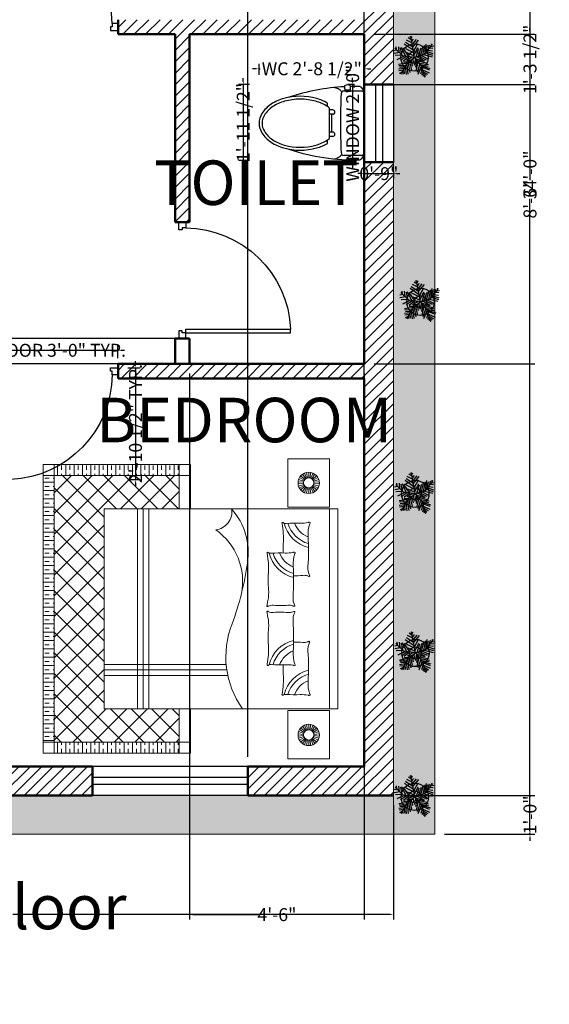
# Model space of a CAD drawing. Units: inches. Extents: x 1265938 to 1266301, y 2357745 to 2358240.
# Tile 2 of 4: x 1266131 to 1266295, y 2357745 to 2358050. Entities that reach past the tile are written whole.
import ezdxf

# ---------------------------------------------------------------- set-up
doc = ezdxf.new("R2010")
doc.units = ezdxf.units.IN
doc.header["$MEASUREMENT"] = 0
for name, color, linetype, lineweight in [('A-ANNO-TEXT', 7, 'Continuous', 25), ('A-AREA-IDEN', 7, 'Continuous', 18), ('A-DOOR', 4, 'Continuous', 25), ('A-FLOR-FIXT', 9, 'Continuous', 25), ('A-FURN', 8, 'Continuous', 18), ('A-WALL-PATT', 8, 'Continuous', 13), ('L-PLNT', 3, 'Continuous', 18), ('L-PLNT-BEDS', 3, 'Continuous', 18), ('L-PLNT-PATT', 3, 'Continuous', 13), ('WALL', 7, 'Continuous', 50), ('WINDOW', 2, 'Continuous', 25), ('YQ_DIM', 3, 'Continuous', 18)]:
    doc.layers.add(name, color=color, linetype=linetype, lineweight=lineweight)
doc.layers.add('Layer2', color=102, linetype='Continuous')
doc.layers.add('RAMP SLOPE', color=8, linetype='Continuous')
doc.styles.get("Standard").update_dxf_attribs({"font": 'arial.ttf'})
doc.styles.add('YQ_DIM', font='SUPEROS.SHX', dxfattribs={"width": 0.8, "bigfont": 'HZDX.SHX'})
doc.dimstyles.new('yqi0', dxfattribs={"dimscale": 0, "dimtxt": 4, "dimasz": 1, "dimexe": 1.5, "dimexo": 3, "dimgap": 0.5, "dimtad": 0, "dimdsep": 46, "dimlunit": 4, "dimtxsty": 'Standard', "dimcen": 0, "dimclrd": 256, "dimclre": 256, "dimclrt": 7, "dimadec": 1, "dimazin": 2, "dimtfac": 1, "dimtix": 1, "dimtmove": 2, "dimatfit": 2, "dimfxl": 1, "dimtolj": 1, "dimtzin": 0, "dimarcsym": 0})

# ---------------------------------------------------------------- blocks, each defined once
blk = doc.blocks.new('WD_WIN4')
for p, q in [((-0.5, 0.5), (0.5, 0.5)), ((-0.5, 0.12), (0.5, 0.12)), ((-0.5, -0.12), (0.5, -0.12)), ((-0.5, -0.5), (0.5, -0.5))]:
    blk.add_line(p, q)
blk = doc.blocks.new('DR_D01')
for p, q in [((-0.45, 0.93), (-0.42, 0.93)), ((-0.45, 0.03), (-0.45, 0.93)), ((-0.42, 0.03), (-0.42, 0.93)), ((-0.5, 0.03), (-0.42, 0.03)), ((-0.5, 0.03), (-0.5, -0.03)), ((-0.45, 0.03), (-0.45, 0)), ((-0.45, 0), (-0.435, 0)), ((-0.435, 0), (-0.435, -0.03)), ((0.435, 0), (0.435, -0.03)), ((0.45, 0), (0.435, 0)), ((0.45, 0.03), (0.45, 0)), ((0.5, 0.03), (0.45, 0.03)), ((0.5, -0.03), (0.5, 0.03)), ((-0.435, -0.03), (-0.5, -0.03)), ((0.435, -0.03), (0.5, -0.03))]:
    blk.add_line(p, q)
blk.add_arc((-0.4602, 0.0206), 0.9103, 0.59152, 87.46644)
blk = doc.blocks.new('Trees - Metric')
at = {"layer": 'Layer2'}
for p, q in [((-258.7244, 1362.456), (-332.3336, 1421.4348)), ((0, 0), (-266.7, 1447.8)), ((-231.1146, 1315.2628), (-166.7002, 1421.4348)), ((-1234.059, 536.7274), (-1252.4486, 737.2604)), ((-1105.2302, 725.4494), (-1077.6458, 395.1732)), ((-902.8176, 713.6638), (-617.5756, 100.2538)), ((-93.091, 489.5342), (-700.3796, 902.3858)), ((-129.8956, 713.6638), (-626.7704, 1032.1544)), ((-185.1152, 1008.5578), (-553.1612, 1185.4942)), ((-221.9198, 1197.3052), (-433.5526, 1338.8594)), ((-194.31, 1102.9442), (-65.4812, 1256.284)), ((-148.3106, 914.1968), (118.5418, 1220.9018)), ((-129.8956, 701.8528), (265.7602, 1185.4942)), ((-74.7014, 418.7444), (219.7608, 961.39)), ((-28.6766, 171.0436), (228.9556, 678.2816)), ((412.9786, 147.447), (587.8068, 796.2392)), ((560.197, 182.8292), (698.2206, 819.8358)), ((685.8, 228.6), (1219.2, 914.4)), ((689.0258, 230.0224), (790.2448, 914.1968)), ((808.6344, 784.4282), (827.0494, 418.7444)), ((891.4384, 831.6214), (946.658, 572.1096)), ((983.4626, 867.0036), (1066.2666, 725.4494)), ((1112.2914, 760.8316), (1296.3144, 784.4282)), ((1121.4862, 925.9824), (1149.0706, 831.6214)), ((-1206.4492, 501.3198), (-1418.082, 465.9376)), ((-1031.621, 347.98), (-1399.667, 277.1902)), ((-800.1, 114.3), (-1333.5, 647.7)), ((-847.598, 159.2326), (-1326.0578, 135.636)), ((-718.7946, 88.4682), (-1215.644, -147.447)), ((-976.4268, 666.4706), (-884.4026, 194.6402)), ((-543.9664, 76.6572), (-967.2066, -206.4512)), ((0, 0), (-800.1, 114.3)), ((-369.1382, 53.086), (-783.1836, 642.874)), ((-405.9428, 53.086), (-764.794, -241.8334)), ((-617.5756, 607.4918), (-74.7014, 347.98)), ((0, 0), (-571.5, -495.3)), ((-166.7002, 29.4894), (-543.9664, -206.4512)), ((-525.5514, 347.98), (-28.6766, 123.8504)), ((0, 0), (685.8, 228.6)), ((0, 0), (457.2, -571.5)), ((100.1268, 41.275), (284.1498, 619.2774)), ((164.5412, 41.275), (661.416, -218.2368)), ((256.5654, 88.4682), (449.7832, 666.4706)), ((284.1498, 88.4682), (781.0246, -147.447)), ((458.978, 147.447), (891.4384, -88.4682)), ((615.4166, 194.6402), (1185.8752, 41.275)), ((753.4148, 312.5978), (1222.6798, 159.2326)), ((845.439, 418.7444), (1241.0948, 277.1902)), ((919.0482, 501.3198), (1222.6798, 454.152)), ((1029.462, 654.685), (1241.0948, 631.0884)), ((-442.7474, -383.3876), (-1086.8406, -477.7486)), ((-617.5756, -548.5384), (-1077.6458, -560.324)), ((-681.9646, -666.496), (-1022.4262, -654.685)), ((-571.5, -495.3), (-952.5, -1143)), ((-387.5278, -324.4088), (-764.794, -324.4088)), ((-635.9652, -607.5172), (-580.771, -1150.1374)), ((-525.5514, -465.963), (-451.9422, -1126.5408)), ((-166.7002, -147.447), (-507.1618, -253.619)), ((-433.5526, -383.3876), (-323.1134, -1020.3688)), ((-341.5284, -289.0012), (-221.9198, -831.6214)), ((-240.3094, -218.2368), (-157.5054, -595.7062)), ((-120.7008, -88.4682), (-93.091, -371.5766)), ((63.3222, -76.6826), (-37.8714, -513.1308)), ((44.9326, -64.897), (615.4166, -241.8334)), ((127.7366, -159.258), (54.1274, -654.685)), ((228.9556, -289.0012), (90.932, -914.1968)), ((357.759, -430.5554), (164.5412, -1020.3688)), ((192.151, -230.0224), (817.8292, -371.5766)), ((458.978, -572.1096), (210.5406, -1161.923)), ((311.7596, -383.3876), (937.4378, -477.7486)), ((412.9786, -501.3452), (919.0482, -583.9206)), ((457.2, -571.5), (685.8, -1333.5)), ((468.1982, -572.1096), (1029.462, -737.2604)), ((486.5878, -642.8994), (983.4626, -843.4324)), ((-718.7946, -737.2604), (-1086.8406, -796.2392)), ((-783.1836, -867.029), (-1077.6458, -902.4112)), ((-875.2078, -1008.5832), (-1040.8412, -1079.3476)), ((-829.2084, -937.7934), (-810.7934, -1126.5408)), ((-737.1842, -784.4536), (-709.5744, -1114.7298)), ((514.1976, -772.6426), (403.7838, -1138.3264)), ((578.612, -961.39), (495.7826, -1232.7128)), ((541.8074, -831.6214), (992.6574, -1032.1544)), ((578.612, -973.1756), (873.0488, -1138.3264)), ((624.6114, -1161.923), (587.8068, -1291.6916)), ((624.6114, -1102.9442), (781.0246, -1209.1162)), ((679.8056, -1268.095), (716.6102, -1291.6916))]:
    blk.add_line(p, q, dxfattribs=at)
blk = doc.blocks.new('A$Cbdbf8f2b')
at = {"layer": 'RAMP SLOPE'}
for radius in [7.17, 3.22]:
    blk.add_circle((13.77, 14.11), radius, dxfattribs=at)
at = {"xscale": 0.0077264756515533, "yscale": 0.0077264756515533, "zscale": 0.0077264756515533}
blk.add_blockref('Trees - Metric', (13.77, 14.11), dxfattribs=at)
blk = doc.blocks.new('BED')
h = blk.add_hatch()
h.set_pattern_fill('TRANS', color=256, scale=12, style=0)
h.set_pattern_definition([(360, (4433.967, -9715.0492), (1e-15, 3), []), (360, (4433.967, -9713.5492), (1e-15, 3), [1.5, -1.5])])
h.paths.add_polyline_path([(48, -103), (52, -103), (52, -58), (48, -58)])
h.paths.add_polyline_path([(-48, -58), (-52, -58), (-52, -103), (-48, -103)])
h = blk.add_hatch()
h.set_pattern_fill('ANSI37', color=256, scale=42, angle=-90, style=0)
h.set_pattern_definition([(315, (7787.1367, 4477.8466), (3.7123106, 3.7123106), []), (45, (7787.1367, 4477.8466), (-3.7123106, 3.7123106), [])])
h.paths.add_polyline_path([(-36, -85), (-36, -58), (-48, -58), (-48, -103), (48, -103), (48, -58), (36, -58), (36, -85)])
h = blk.add_hatch()
h.set_pattern_fill('TRANS', color=256, scale=12, angle=-90, style=0)
h.set_pattern_definition([(270, (4433.967, -9715.0492), (3, -1e-15), []), (270, (4435.467, -9715.0492), (3, -1e-15), [1.5, -1.5])])
h.paths.add_polyline_path([(48, -107), (48, -103), (-48, -103), (-48, -107)])
for p, q in [((-36, -1), (36, -1)), ((-36, -85), (-36, -1)), ((36, -1), (36, -85)), ((-54, -4), (-54, -19)), ((-36.64, -4), (-54, -4)), ((-36.64, -4), (-36.64, -19)), ((-36, -4), (36, -4)), ((36.64, -4), (36.64, -19)), ((36.64, -4), (54, -4)), ((54, -4), (54, -19)), ((-47.07, -10.7), (-48.9, -9.89)), ((-46.88, -10.37), (-48.5, -9.2)), ((-46.62, -10.08), (-47.96, -8.6)), ((-46.31, -9.86), (-47.31, -8.13)), ((-45.96, -9.7), (-46.58, -7.8)), ((-45.58, -9.62), (-45.8, -7.63)), ((-45.2, -9.62), (-45, -7.63)), ((-44.82, -9.7), (-44.21, -7.79)), ((-44.47, -9.85), (-43.48, -8.12)), ((-44.16, -10.08), (-42.83, -8.59)), ((-43.9, -10.36), (-42.29, -9.18)), ((-43.71, -10.7), (-41.89, -9.88)), ((43.71, -10.7), (41.89, -9.88)), ((43.9, -10.36), (42.29, -9.18)), ((44.16, -10.08), (42.83, -8.59)), ((44.47, -9.85), (43.48, -8.12)), ((44.82, -9.7), (44.21, -7.79)), ((45.2, -9.62), (45, -7.63)), ((45.58, -9.62), (45.8, -7.63)), ((45.96, -9.7), (46.58, -7.8)), ((46.31, -9.86), (47.31, -8.13)), ((46.62, -10.08), (47.96, -8.6)), ((46.88, -10.37), (48.5, -9.2)), ((47.07, -10.7), (48.9, -9.89)), ((-47.23, -11.45), (-49.23, -11.45)), ((-47.19, -11.07), (-49.14, -10.66)), ((-47.19, -11.83), (-49.14, -12.25)), ((-47.07, -12.2), (-48.89, -13.01)), ((-46.87, -12.53), (-48.49, -13.71)), ((-46.62, -12.81), (-47.95, -14.3)), ((-46.3, -13.04), (-47.3, -14.77)), ((-45.95, -13.2), (-46.57, -15.1)), ((-45.58, -13.27), (-45.78, -15.26)), ((-45.19, -13.27), (-44.98, -15.26)), ((-44.82, -13.19), (-44.2, -15.09)), ((-44.47, -13.04), (-43.46, -14.77)), ((-44.16, -12.81), (-42.82, -14.29)), ((-43.9, -12.52), (-42.28, -13.7)), ((-43.71, -12.19), (-41.88, -13)), ((-43.59, -11.06), (-41.64, -10.64)), ((-43.59, -11.83), (-41.63, -12.24)), ((-43.55, -11.44), (-41.55, -11.44)), ((43.55, -11.44), (41.55, -11.44)), ((43.59, -11.83), (41.63, -12.24)), ((43.59, -11.06), (41.64, -10.64)), ((43.71, -12.19), (41.88, -13)), ((43.9, -12.52), (42.28, -13.7)), ((44.16, -12.81), (42.82, -14.29)), ((44.47, -13.04), (43.46, -14.77)), ((44.82, -13.19), (44.2, -15.09)), ((45.19, -13.27), (44.98, -15.26)), ((45.58, -13.27), (45.78, -15.26)), ((45.95, -13.2), (46.57, -15.1)), ((46.3, -13.04), (47.3, -14.77)), ((46.62, -12.81), (47.95, -14.3)), ((46.87, -12.53), (48.49, -13.71)), ((47.07, -12.2), (48.89, -13.01)), ((47.19, -11.07), (49.14, -10.66)), ((47.19, -11.83), (49.14, -12.25)), ((47.23, -11.45), (49.23, -11.45)), ((-36.64, -19), (-54, -19)), ((36.64, -19), (54, -19)), ((20, -85), (20, -41.14)), ((22, -85), (22, -40.91)), ((24, -85), (24, -40.55)), ((-52, -54), (-52, -107)), ((-52, -54), (-36, -54)), ((-48, -54), (-48, -107)), ((36, -54), (52, -54)), ((48, -54), (48, -107)), ((52, -54), (52, -107)), ((-52, -58), (-36, -58)), ((36, -58), (52, -58)), ((36, -69), (-36, -69)), ((36, -71), (-36, -71)), ((36, -73), (-36, -73)), ((36, -85), (-36, -85)), ((-52, -103), (52, -103)), ((-52, -107), (52, -107))]:
    blk.add_line(p, q)
for centre, radius in [((-45.39, -11.45), 3.84), ((-45.39, -11.45), 1.84), ((45.39, -11.45), 3.84), ((45.39, -11.45), 1.84)]:
    blk.add_circle(centre, radius)
for centre, radius, start, end in [((-30.92, -11.24), 0.328, 35.8976, 208.6272), ((-42.38, -17.5), 12.73, 27.1629, 28.6272), ((-44.37, -13.89), 13.5, 357.4804, 9.3956), ((-33.8, -8.61), 8.46, 289.8695, 338.9843), ((-33.8, -8.61), 12.06, 283.8498, 346.0842), ((-33.8, -8.61), 10.71, 286.0319, 344.1205), ((-26.84, 0.13), 11.82, 251.1782, 273.3982), ((-20.92, -99.64), 88.13, 86.2964, 93.3982), ((-14.79, -4.98), 6.73, 266.2964, 294.303), ((-8.24, -13.16), 3.86, 159.0146, 186.273), ((-36.64, -16.28), 24.71, 358.5721, 6.273), ((-11.92, -11.33), 0.242, 335.7259, 114.303), ((-5.69, -14.14), 6.59, 155.7259, 159.0146), ((11.92, -11.33), 0.242, 65.697, 204.2741), ((5.69, -14.14), 6.59, 20.9854, 24.2741), ((8.24, -13.16), 3.86, 353.727, 20.9854), ((36.64, -16.28), 24.71, 173.727, 181.4279), ((14.79, -4.98), 6.73, 245.697, 273.7036), ((20.92, -99.64), 88.13, 86.6018, 93.7036), ((33.8, -8.61), 12.06, 193.9158, 256.1502), ((33.8, -8.61), 10.71, 195.8795, 253.9681), ((33.8, -8.61), 8.46, 201.0157, 250.1305), ((26.84, 0.13), 11.82, 266.6018, 288.8218), ((30.92, -11.24), 0.328, 331.3728, 144.1024), ((44.37, -13.89), 13.5, 170.6044, 182.5196), ((42.38, -17.5), 12.73, 151.3728, 152.8371), ((10.15, -16.29), 41.07, 177.4804, 184.5075), ((-20.16, -16.62), 0.328, 35.8976, 208.6272), ((-31.62, -22.87), 12.73, 27.1629, 28.6272), ((-33.61, -19.26), 13.5, 357.4804, 9.3956), ((-23.04, -13.99), 8.46, 289.8695, 338.9843), ((-23.04, -13.99), 12.06, 283.8498, 346.0842), ((-23.04, -13.99), 10.71, 286.0319, 344.1205), ((-16.08, -5.24), 11.82, 251.1782, 273.3982), ((-10.15, -105.01), 88.13, 86.2964, 93.3982), ((-4.03, -10.35), 6.73, 266.2964, 294.303), ((2.52, -18.53), 3.86, 159.0146, 186.273), ((-1.16, -16.7), 0.242, 335.7259, 114.303), ((5.07, -19.51), 6.59, 155.7259, 159.0146), ((1.16, -16.7), 0.242, 65.697, 204.2741), ((-5.07, -19.51), 6.59, 20.9854, 24.2741), ((-2.52, -18.53), 3.86, 353.727, 20.9854), ((4.03, -10.35), 6.73, 245.697, 273.7036), ((10.15, -105.01), 88.13, 86.6018, 93.7036), ((23.04, -13.99), 12.06, 193.9158, 256.1502), ((23.04, -13.99), 10.71, 195.8795, 253.9681), ((23.04, -13.99), 8.46, 201.0157, 250.1305), ((16.08, -5.24), 11.82, 266.6018, 288.8218), ((20.16, -16.62), 0.328, 331.3728, 144.1024), ((33.61, -19.26), 13.5, 170.6044, 182.5196), ((31.62, -22.87), 12.73, 151.3728, 152.8371), ((-10.15, -16.29), 41.07, 355.4925, 2.5196), ((-30.88, -20.82), 0.25, 147.6219, 311.9343), ((-32.72, -19.65), 1.93, 327.6219, 339.2246), ((-32.67, -19.67), 1.88, 339.2246, 4.5075), ((-25.16, -53.53), 33, 93.5164, 99.6766), ((-25.27, -51.86), 31.33, 86.4836, 93.5164), ((-21.12, 15.68), 36.34, 266.4836, 271.5234), ((20.91, -21.66), 41.07, 177.4804, 184.5075), ((-25.88, -21.66), 24.71, 354.3784, 6.273), ((25.88, -21.66), 24.71, 173.727, 185.6216), ((-20.91, -21.66), 41.07, 355.4925, 2.5196), ((21.12, 15.68), 36.34, 268.4766, 273.5164), ((25.27, -51.86), 31.33, 86.4836, 93.5164), ((25.16, -53.53), 33, 80.3234, 86.4836), ((30.88, -20.82), 0.25, 228.0657, 32.3781), ((32.67, -19.67), 1.88, 175.4925, 200.7754), ((32.72, -19.65), 1.93, 200.7754, 212.3781), ((2.55, -24.46), 3.86, 174.3784, 204.7617), ((-2.55, -24.46), 3.86, 335.2383, 5.6216), ((-20.12, -26.19), 0.25, 147.6219, 311.9343), ((-21.96, -25.02), 1.93, 327.6219, 339.2246), ((-21.91, -25.04), 1.88, 339.2246, 4.5075), ((-14.4, -58.9), 33, 93.5164, 99.6766), ((-14.51, -57.23), 31.33, 86.4836, 93.5164), ((-10.35, 10.3), 36.34, 266.4836, 275.306), ((-5.78, -38.98), 13.15, 77.9645, 95.306), ((2.5, -0.17), 26.53, 257.9645, 261.9243), ((-1.09, -26.25), 0.228, 231.9005, 52.8902), ((1.09, -26.25), 0.228, 127.1098, 308.0995), ((-2.5, -0.17), 26.53, 278.0757, 282.0355), ((5.78, -38.98), 13.15, 84.694, 102.0355), ((10.35, 10.3), 36.34, 264.694, 273.5164), ((14.51, -57.23), 31.33, 86.4836, 93.5164), ((14.4, -58.9), 33, 80.3234, 86.4836), ((20.12, -26.19), 0.25, 228.0657, 32.3781), ((21.91, -25.04), 1.88, 175.4925, 200.7754), ((21.96, -25.02), 1.93, 200.7754, 212.3781), ((-20.27, -56.85), 23.66, 81.0857, 131.6581), ((-9.91, -57.83), 22.61, 78.6456, 145.1521), ((-32.56, -143.87), 111.55, 70.0977, 81.7735), ((17.27, -9.21), 32.05, 248.2778, 305.7663), ((-34.97, -45.63), 6.55, 6.3172, 99.0807)]:
    blk.add_arc(centre, radius, start, end)
blk = doc.blocks.new('yq_matong_01')
for p, q in [((20, 220.5), (138.8, 220.5)), ((0, 200.5), (0, -200.5)), ((252.5, 138), (252.5, 114.5)), ((215.8, 91), (238, 91)), ((238, 104.1), (238, -104.1)), ((215.8, 61), (238, 61)), ((223, 61), (223, -61)), ((215.8, -61), (238, -61)), ((215.8, -91), (238, -91)), ((252.5, -114.5), (252.5, -138)), ((20, -220.5), (138.8, -220.5)), ((97.4, -220.5), (97.4, -225.5)), ((97.4, -225.5), (131.6, -225.5)), ((131.6, -220.5), (131.6, -225.5))]:
    blk.add_line(p, q)
for centre, radius, start, end in [((54.8, 202.4), 54.8, 117.32201, 181.89921), ((20, 200.5), 20, 90, 180), ((63.9, -1165.4), 1416.8, 71.40679, 91.38565), ((138.8, 200.5), 20, 2.30634, 90), ((216.6, 161.2), 83.2, 95.49628, 139.93242), ((-4840.4, 0), 5003.3, 357.69366, 2.30634), ((406.6, -122.9), 283, 105.20877, 123.27785), ((406.6, -122.9), 303, 105.20877, 120.56985), ((439, -242.2), 426.7, 74.79123, 105.20877), ((439, -242.2), 406.7, 74.79123, 105.20877), ((471.4, -122.9), 283, 56.72215, 74.79123), ((471.4, -122.9), 303, 56.72215, 74.79123), ((215.8, 76), 15, 90, 270), ((357.1, -47.5), 192.8, 123.27785, 128.13838), ((520.9, -47.5), 192.8, 32.25649, 56.72215), ((520.9, -47.5), 212.8, 32.25649, 56.72215), ((596.2, 0), 103.8, 360, 32.25649), ((596.2, 0), 123.8, 360, 32.25649), ((215.8, -76), 15, 90, 270), ((520.9, 47.5), 192.8, 303.27785, 327.74351), ((520.9, 47.5), 212.8, 303.27785, 327.74351), ((596.2, 0), 103.8, 327.74351, 360), ((596.2, 0), 123.8, 327.74351, 360), ((357.1, 47.5), 192.8, 231.86162, 236.72215), ((406.6, 122.9), 283, 236.72215, 254.79123), ((471.4, 122.9), 283, 285.20877, 303.27785), ((471.4, 122.9), 303, 285.20877, 303.27785), ((51.3, -204.4), 51.4, 175.68696, 245.09182), ((20, -200.5), 20, 180, 270), ((63.9, 1165.4), 1416.8, 272.89667, 288.59321), ((138.8, -200.5), 20, 270, 357.69366), ((406.6, 122.9), 303, 239.43015, 254.79123), ((439, 242.2), 426.7, 254.79123, 285.20877), ((439, 242.2), 406.7, 254.79123, 285.20877), ((63.9, 1165.4), 1416.8, 268.61435, 271.20362), ((156.6, -247.4), 63.1, 159.68336, 188.49388), ((114.1, -225.6), 37, 237.52867, 304.27722), ((72.4, -247.4), 63.1, 352.09441, 20.31664), ((216.6, -161.2), 83.2, 220.06758, 264.50372)]:
    blk.add_arc(centre, radius, start, end)
blk = doc.blocks.new('*D24')
at = {"layer": 'Defpoints', "color": 0, "transparency": 16777216}
for p in [(1266237.39, 2358029.66), (1266233.79, 2358005.66), (1266237.39, 2358005.66)]:
    blk.add_point(p, dxfattribs=at)
at = {"layer": 'YQ_DIM', "lineweight": -2, "transparency": 16777216}
for p, q in [((1266234.39, 2358029.66), (1266232.29, 2358029.66)), ((1266233.79, 2358030.66), (1266233.79, 2358031.66)), ((1266233.79, 2358029.66), (1266233.79, 2358005.66)), ((1266234.39, 2358005.66), (1266232.29, 2358005.66)), ((1266233.79, 2358004.66), (1266233.79, 2358003.66))]:
    blk.add_line(p, q, dxfattribs=at)
at = {"layer": 'YQ_DIM', "transparency": 16777216}
for points in [[(1266233.62, 2358030.66), (1266233.96, 2358030.66), (1266233.79, 2358029.66)], [(1266233.62, 2358004.66), (1266233.96, 2358004.66), (1266233.79, 2358005.66)]]:
    blk.add_solid(points, dxfattribs=at)
at = {"layer": 'YQ_DIM', "color": 7, "transparency": 16777216, "insert": (1266233.79, 2358017.66), "char_height": 4, "attachment_point": 5, "rotation": 90}
blk.add_mtext('\\A1;WINDOW 2\'-0"', dxfattribs=at)
blk = doc.blocks.new('*D25')
at = {"layer": 'Defpoints', "color": 0, "transparency": 16777216}
for p in [(1266237.39, 2358005.66), (1266246.39, 2358005.66), (1266246.39, 2358002.06)]:
    blk.add_point(p, dxfattribs=at)
at = {"layer": 'YQ_DIM', "lineweight": -2, "transparency": 16777216}
for p, q in [((1266236.39, 2358002.06), (1266235.39, 2358002.06)), ((1266237.39, 2358002.66), (1266237.39, 2358000.56)), ((1266237.39, 2358002.06), (1266246.39, 2358002.06)), ((1266246.39, 2358002.66), (1266246.39, 2358000.56)), ((1266247.39, 2358002.06), (1266248.39, 2358002.06))]:
    blk.add_line(p, q, dxfattribs=at)
at = {"layer": 'YQ_DIM', "transparency": 16777216}
for points in [[(1266236.39, 2358002.22), (1266236.39, 2358001.89), (1266237.39, 2358002.06)], [(1266247.39, 2358002.22), (1266247.39, 2358001.89), (1266246.39, 2358002.06)]]:
    blk.add_solid(points, dxfattribs=at)
at = {"layer": 'YQ_DIM', "color": 7, "transparency": 16777216, "insert": (1266241.89, 2358002.06), "char_height": 4, "attachment_point": 5}
blk.add_mtext('\\A1;0\'-9"', dxfattribs=at)
blk = doc.blocks.new('*D26')
at = {"layer": 'Defpoints', "color": 0, "transparency": 16777216}
for p in [(1266161.26, 2357947.41), (1266125.26, 2357942.01), (1266161.26, 2357942.01)]:
    blk.add_point(p, dxfattribs=at)
at = {"layer": 'YQ_DIM', "lineweight": -2, "transparency": 16777216}
for p, q in [((1266124.26, 2357947.41), (1266123.26, 2357947.41)), ((1266125.26, 2357945.01), (1266125.26, 2357948.91)), ((1266125.26, 2357947.41), (1266161.26, 2357947.41)), ((1266161.26, 2357945.01), (1266161.26, 2357948.91)), ((1266162.26, 2357947.41), (1266163.26, 2357947.41))]:
    blk.add_line(p, q, dxfattribs=at)
at = {"layer": 'YQ_DIM', "transparency": 16777216}
for points in [[(1266124.26, 2357947.58), (1266124.26, 2357947.24), (1266125.26, 2357947.41)], [(1266162.26, 2357947.58), (1266162.26, 2357947.24), (1266161.26, 2357947.41)]]:
    blk.add_solid(points, dxfattribs=at)
at = {"layer": 'YQ_DIM', "color": 7, "transparency": 16777216, "insert": (1266143.26, 2357947.41), "char_height": 4, "attachment_point": 5}
blk.add_mtext('\\A1;DOOR 3\'-0" TYP.', dxfattribs=at)
blk = doc.blocks.new('*D27')
at = {"layer": 'Defpoints', "color": 0, "transparency": 16777216}
for p in [(1266161.26, 2357942.01), (1266161.26, 2357907.45), (1266166.66, 2357907.45)]:
    blk.add_point(p, dxfattribs=at)
at = {"layer": 'YQ_DIM', "lineweight": -2, "transparency": 16777216}
for p, q in [((1266166.66, 2357943.01), (1266166.66, 2357944.01)), ((1266164.26, 2357942.01), (1266168.16, 2357942.01)), ((1266166.66, 2357942.01), (1266166.66, 2357907.45)), ((1266164.26, 2357907.45), (1266168.16, 2357907.45)), ((1266166.66, 2357906.45), (1266166.66, 2357905.45))]:
    blk.add_line(p, q, dxfattribs=at)
at = {"layer": 'YQ_DIM', "transparency": 16777216}
for points in [[(1266166.5, 2357943.01), (1266166.83, 2357943.01), (1266166.66, 2357942.01)], [(1266166.5, 2357906.45), (1266166.83, 2357906.45), (1266166.66, 2357907.45)]]:
    blk.add_solid(points, dxfattribs=at)
at = {"layer": 'YQ_DIM', "color": 7, "transparency": 16777216, "insert": (1266166.66, 2357924.73), "char_height": 4, "attachment_point": 5, "rotation": 90}
blk.add_mtext('\\A1;2\'-10 1/2" TYP.', dxfattribs=at)
blk = doc.blocks.new('*D28')
at = {"layer": 'Defpoints', "color": 0, "transparency": 16777216}
for p in [(1266204.87, 2358034.5), (1266204.87, 2358029.61), (1266237.46, 2358029.61)]:
    blk.add_point(p, dxfattribs=at)
at = {"layer": 'YQ_DIM', "lineweight": -2, "transparency": 16777216}
for p, q in [((1266204.87, 2358032.61), (1266204.87, 2358036)), ((1266237.46, 2358032.61), (1266237.46, 2358036)), ((1266203.87, 2358034.5), (1266202.87, 2358034.5)), ((1266204.87, 2358034.5), (1266205.18, 2358034.5)), ((1266237.46, 2358034.5), (1266237.16, 2358034.5)), ((1266238.46, 2358034.5), (1266239.46, 2358034.5))]:
    blk.add_line(p, q, dxfattribs=at)
at = {"layer": 'YQ_DIM', "transparency": 16777216}
for points in [[(1266203.87, 2358034.66), (1266203.87, 2358034.33), (1266204.87, 2358034.5)], [(1266238.46, 2358034.66), (1266238.46, 2358034.33), (1266237.46, 2358034.5)]]:
    blk.add_solid(points, dxfattribs=at)
at = {"layer": 'YQ_DIM', "color": 7, "transparency": 16777216, "insert": (1266221.17, 2358034.5), "char_height": 4, "attachment_point": 5}
blk.add_mtext('\\A1;WC 2\'-8 1/2"', dxfattribs=at)
blk = doc.blocks.new('*D29')
at = {"layer": 'Defpoints', "color": 0, "transparency": 16777216}
for p in [(1266204.87, 2358029.61), (1266199.99, 2358006.14), (1266204.87, 2358006.14)]:
    blk.add_point(p, dxfattribs=at)
at = {"layer": 'YQ_DIM', "lineweight": -2, "transparency": 16777216}
for p, q in [((1266201.87, 2358029.61), (1266198.49, 2358029.61)), ((1266199.99, 2358030.61), (1266199.99, 2358031.61)), ((1266199.99, 2358029.61), (1266199.99, 2358006.14)), ((1266201.87, 2358006.14), (1266198.49, 2358006.14)), ((1266199.99, 2358005.14), (1266199.99, 2358004.14))]:
    blk.add_line(p, q, dxfattribs=at)
at = {"layer": 'YQ_DIM', "transparency": 16777216}
for points in [[(1266199.82, 2358030.61), (1266200.15, 2358030.61), (1266199.99, 2358029.61)], [(1266199.82, 2358005.14), (1266200.15, 2358005.14), (1266199.99, 2358006.14)]]:
    blk.add_solid(points, dxfattribs=at)
at = {"layer": 'YQ_DIM', "color": 7, "transparency": 16777216, "insert": (1266199.99, 2358017.87), "char_height": 4, "attachment_point": 5, "rotation": 90}
blk.add_mtext('\\A1;1\'-11 1/2"', dxfattribs=at)
blk = doc.blocks.new('*D35')
at = {"layer": 'Defpoints', "color": 0, "transparency": 16777216}
for p in [(1266259.14, 2358205.68), (1266288.6, 2358205.68), (1266259.14, 2357797.68)]:
    blk.add_point(p, dxfattribs=at)
at = {"layer": 'YQ_DIM', "lineweight": -2, "transparency": 16777216}
for p, q in [((1266262.14, 2358205.68), (1266290.1, 2358205.68)), ((1266288.6, 2358204.68), (1266288.6, 2358009.05)), ((1266288.6, 2357798.68), (1266288.6, 2357994.31)), ((1266262.14, 2357797.68), (1266290.1, 2357797.68))]:
    blk.add_line(p, q, dxfattribs=at)
at = {"layer": 'YQ_DIM', "transparency": 16777216}
for points in [[(1266288.44, 2358204.68), (1266288.77, 2358204.68), (1266288.6, 2358205.68)], [(1266288.44, 2357798.68), (1266288.77, 2357798.68), (1266288.6, 2357797.68)]]:
    blk.add_solid(points, dxfattribs=at)
at = {"layer": 'YQ_DIM', "color": 7, "transparency": 16777216, "insert": (1266288.6, 2358001.68), "char_height": 4, "attachment_point": 5, "rotation": 90}
blk.add_mtext('\\A1;34\'-0"', dxfattribs=at)
blk = doc.blocks.new('*D36')
at = {"layer": 'Defpoints', "color": 0, "transparency": 16777216}
for p in [(1265983.89, 2357809.68), (1266246.39, 2357809.68), (1266246.39, 2357772.83)]:
    blk.add_point(p, dxfattribs=at)
at = {"layer": 'YQ_DIM', "lineweight": -2, "transparency": 16777216}
for p, q in [((1265983.89, 2357806.68), (1265983.89, 2357771.33)), ((1266246.39, 2357806.68), (1266246.39, 2357771.33)), ((1265984.89, 2357772.83), (1266101.52, 2357772.83)), ((1266245.39, 2357772.83), (1266128.76, 2357772.83))]:
    blk.add_line(p, q, dxfattribs=at)
at = {"layer": 'YQ_DIM', "transparency": 16777216}
for points in [[(1265984.89, 2357773), (1265984.89, 2357772.66), (1265983.89, 2357772.83)], [(1266245.39, 2357773), (1266245.39, 2357772.66), (1266246.39, 2357772.83)]]:
    blk.add_solid(points, dxfattribs=at)
at = {"layer": 'YQ_DIM', "color": 7, "transparency": 16777216, "insert": (1266115.14, 2357772.83), "char_height": 4, "attachment_point": 5}
blk.add_mtext('\\A1;21\'-10 1/2"', dxfattribs=at)
blk = doc.blocks.new('*D40')
at = {"layer": 'Defpoints', "color": 0, "transparency": 16777216}
for p in [(1266237.39, 2358045.18), (1266288.6, 2358045.18), (1266237.39, 2357943.18)]:
    blk.add_point(p, dxfattribs=at)
at = {"layer": 'YQ_DIM', "lineweight": -2, "transparency": 16777216}
for p, q in [((1266240.39, 2358045.18), (1266290.1, 2358045.18)), ((1266288.6, 2358044.18), (1266288.6, 2358000)), ((1266288.6, 2357944.18), (1266288.6, 2357988.36)), ((1266240.39, 2357943.18), (1266290.1, 2357943.18))]:
    blk.add_line(p, q, dxfattribs=at)
at = {"layer": 'YQ_DIM', "transparency": 16777216}
for points in [[(1266288.44, 2358044.18), (1266288.77, 2358044.18), (1266288.6, 2358045.18)], [(1266288.44, 2357944.18), (1266288.77, 2357944.18), (1266288.6, 2357943.18)]]:
    blk.add_solid(points, dxfattribs=at)
at = {"layer": 'YQ_DIM', "color": 7, "transparency": 16777216, "insert": (1266288.6, 2357994.18), "char_height": 4, "attachment_point": 5, "rotation": 90}
blk.add_mtext('\\A1;8\'-6"', dxfattribs=at)
blk = doc.blocks.new('*D41')
at = {"layer": 'Defpoints', "color": 0, "transparency": 16777216}
for p in [(1266183.39, 2357943.18), (1266237.39, 2357943.18), (1266237.39, 2357772.83)]:
    blk.add_point(p, dxfattribs=at)
at = {"layer": 'YQ_DIM', "lineweight": -2, "transparency": 16777216}
for p, q in [((1266183.39, 2357940.18), (1266183.39, 2357771.33)), ((1266237.39, 2357940.18), (1266237.39, 2357771.33)), ((1266184.39, 2357772.83), (1266204.49, 2357772.83)), ((1266236.39, 2357772.83), (1266216.29, 2357772.83))]:
    blk.add_line(p, q, dxfattribs=at)
at = {"layer": 'YQ_DIM', "transparency": 16777216}
for points in [[(1266184.39, 2357773), (1266184.39, 2357772.66), (1266183.39, 2357772.83)], [(1266236.39, 2357773), (1266236.39, 2357772.66), (1266237.39, 2357772.83)]]:
    blk.add_solid(points, dxfattribs=at)
at = {"layer": 'YQ_DIM', "color": 7, "transparency": 16777216, "insert": (1266210.39, 2357772.83), "char_height": 4, "attachment_point": 5}
blk.add_mtext('\\A1;4\'-6"', dxfattribs=at)
blk = doc.blocks.new('*D46')
at = {"layer": 'Defpoints', "color": 0, "transparency": 16777216}
for p in [(1266237.39, 2358045.18), (1266237.39, 2358029.66), (1266288.6, 2358029.66)]:
    blk.add_point(p, dxfattribs=at)
at = {"layer": 'YQ_DIM', "lineweight": -2, "transparency": 16777216}
for p, q in [((1266240.39, 2358045.18), (1266290.1, 2358045.18)), ((1266288.6, 2358046.18), (1266288.6, 2358047.18)), ((1266288.6, 2358045.18), (1266288.6, 2358029.66)), ((1266240.39, 2358029.66), (1266290.1, 2358029.66)), ((1266288.6, 2358028.66), (1266288.6, 2358027.66))]:
    blk.add_line(p, q, dxfattribs=at)
at = {"layer": 'YQ_DIM', "transparency": 16777216}
for points in [[(1266288.44, 2358046.18), (1266288.77, 2358046.18), (1266288.6, 2358045.18)], [(1266288.44, 2358028.66), (1266288.77, 2358028.66), (1266288.6, 2358029.66)]]:
    blk.add_solid(points, dxfattribs=at)
at = {"layer": 'YQ_DIM', "color": 7, "transparency": 16777216, "insert": (1266288.6, 2358037.42), "char_height": 4, "attachment_point": 5, "rotation": 90}
blk.add_mtext('\\A1;1\'-3 1/2"', dxfattribs=at)
blk = doc.blocks.new('*D47')
at = {"layer": 'Defpoints', "color": 0, "transparency": 16777216}
for p in [(1266201.39, 2358237.77), (1266201.39, 2357818.68), (1266237.39, 2357818.68)]:
    blk.add_point(p, dxfattribs=at)
at = {"layer": 'YQ_DIM', "lineweight": -2, "transparency": 16777216}
for p, q in [((1266201.39, 2357821.68), (1266201.39, 2358239.27)), ((1266237.39, 2357821.68), (1266237.39, 2358239.27)), ((1266202.39, 2358237.77), (1266213.58, 2358237.77)), ((1266236.39, 2358237.77), (1266225.21, 2358237.77))]:
    blk.add_line(p, q, dxfattribs=at)
at = {"layer": 'YQ_DIM', "transparency": 16777216}
for points in [[(1266202.39, 2358237.93), (1266202.39, 2358237.6), (1266201.39, 2358237.77)], [(1266236.39, 2358237.93), (1266236.39, 2358237.6), (1266237.39, 2358237.77)]]:
    blk.add_solid(points, dxfattribs=at)
at = {"layer": 'YQ_DIM', "color": 7, "transparency": 16777216, "insert": (1266219.39, 2358237.77), "char_height": 4, "attachment_point": 5}
blk.add_mtext('\\A1;3\'-0"', dxfattribs=at)
blk = doc.blocks.new('*D50')
at = {"layer": 'Defpoints', "color": 0, "transparency": 16777216}
for p in [(1265944.45, 2357951.05), (1266183.39, 2357951.05), (1266183.39, 2357943.18)]:
    blk.add_point(p, dxfattribs=at)
at = {"layer": 'YQ_DIM', "lineweight": -2, "transparency": 16777216}
for p, q in [((1265944.45, 2357952.05), (1265944.45, 2357953.05)), ((1266180.39, 2357951.05), (1265942.95, 2357951.05)), ((1265944.45, 2357943.18), (1265944.45, 2357951.05)), ((1266180.39, 2357943.18), (1265942.95, 2357943.18)), ((1265944.45, 2357942.18), (1265944.45, 2357941.18))]:
    blk.add_line(p, q, dxfattribs=at)
at = {"layer": 'YQ_DIM', "transparency": 16777216}
for points in [[(1265944.29, 2357952.05), (1265944.62, 2357952.05), (1265944.45, 2357951.05)], [(1265944.29, 2357942.18), (1265944.62, 2357942.18), (1265944.45, 2357943.18)]]:
    blk.add_solid(points, dxfattribs=at)
at = {"layer": 'YQ_DIM', "color": 7, "transparency": 16777216, "insert": (1265944.45, 2357947.12), "char_height": 4, "attachment_point": 5, "rotation": 90}
blk.add_mtext('\\A1;0\'-8"', dxfattribs=at)
blk = doc.blocks.new('*D58')
at = {"layer": 'Defpoints', "color": 0, "transparency": 16777216}
for p in [(1266246.39, 2357809.68), (1266288.6, 2357809.68), (1266259.14, 2357797.68)]:
    blk.add_point(p, dxfattribs=at)
at = {"layer": 'YQ_DIM', "lineweight": -2, "transparency": 16777216}
for p, q in [((1266288.6, 2357810.68), (1266288.6, 2357811.68)), ((1266249.39, 2357809.68), (1266290.1, 2357809.68)), ((1266288.6, 2357809.68), (1266288.6, 2357809.31)), ((1266262.14, 2357797.68), (1266290.1, 2357797.68)), ((1266288.6, 2357797.68), (1266288.6, 2357798.05)), ((1266288.6, 2357796.68), (1266288.6, 2357795.68))]:
    blk.add_line(p, q, dxfattribs=at)
at = {"layer": 'YQ_DIM', "transparency": 16777216}
for points in [[(1266288.44, 2357810.68), (1266288.77, 2357810.68), (1266288.6, 2357809.68)], [(1266288.44, 2357796.68), (1266288.77, 2357796.68), (1266288.6, 2357797.68)]]:
    blk.add_solid(points, dxfattribs=at)
at = {"layer": 'YQ_DIM', "color": 7, "transparency": 16777216, "insert": (1266288.6, 2357803.68), "char_height": 4, "attachment_point": 5, "rotation": 90}
blk.add_mtext('\\A1;1\'-0"', dxfattribs=at)

msp = doc.modelspace()

# ---------------------------------------------------------------- hatches: boundary and pattern name
at = {"layer": 'A-WALL-PATT'}
h = msp.add_hatch(dxfattribs=at)
h.set_pattern_fill('ANSI31', color=256, scale=20)
h.paths.add_polyline_path([(1266069.016, 2358049.681), (1265992.89, 2358049.681), (1265992.89, 2358099.181), (1265983.89, 2358099.181), (1265983.89, 2358012.181), (1265992.89, 2358012.181), (1265992.89, 2358045.181), (1266069.016, 2358045.181)])
h.paths.add_polyline_path([(1266246.39, 2358049.681), (1266246.39, 2358099.181), (1266237.39, 2358099.181), (1266237.39, 2358049.681), (1266161.264, 2358049.681), (1266161.264, 2358045.181), (1266178.89, 2358045.181), (1266178.89, 2357987.055), (1266183.39, 2357987.055), (1266183.39, 2358045.181), (1266237.39, 2358045.181), (1266237.39, 2358029.655), (1266246.39, 2358029.655)])
h.paths.add_polyline_path([(1265992.89, 2357938.681), (1266058.89, 2357938.681), (1266058.89, 2357943.181), (1265992.89, 2357943.181), (1265992.89, 2357976.181), (1265983.89, 2357976.181), (1265983.89, 2357967.701), (1265984.307, 2357966.989), (1265983.89, 2357967.035), (1265983.89, 2357902.681), (1265992.89, 2357902.681)])
h.paths.add_polyline_path([(1266069.016, 2357943.181), (1266058.89, 2357943.181), (1266058.89, 2357938.681), (1266069.016, 2357938.681)])
h.paths.add_polyline_path([(1266125.264, 2357943.181), (1266105.016, 2357943.181), (1266105.016, 2357938.681), (1266112.89, 2357938.681), (1266112.89, 2357818.681), (1266105.024, 2357818.681), (1266105.024, 2357809.681), (1266112.898, 2357809.681), (1266153.39, 2357809.681), (1266153.39, 2357818.681), (1266117.39, 2357818.681), (1266117.39, 2357938.681), (1266125.264, 2357938.681)])
h.paths.add_polyline_path([(1266069.024, 2357818.681), (1265999.055, 2357818.681), (1265992.89, 2357818.681), (1265992.89, 2357854.681), (1265983.89, 2357854.681), (1265983.89, 2357809.681), (1266069.024, 2357809.681)])
h.paths.add_polyline_path([(1266246.39, 2358005.655), (1266237.39, 2358005.655), (1266237.39, 2357943.181), (1266161.264, 2357943.181), (1266161.264, 2357938.681), (1266237.39, 2357938.681), (1266237.39, 2357818.681), (1266201.39, 2357818.681), (1266201.39, 2357809.681), (1266246.39, 2357809.681)])
at = {"layer": 'L-PLNT-PATT'}
h = msp.add_hatch(dxfattribs=at)
h.set_pattern_fill('GRASS', color=256, scale=4)
h.paths.add_polyline_path([(1266259.14, 2358205.681), (1266246.39, 2358205.681), (1266246.39, 2358099.181), (1266246.39, 2358049.681), (1266246.39, 2357797.681), (1266259.14, 2357797.681), (1266259.14, 2358049.681)])
h = msp.add_hatch(dxfattribs=at)
h.set_pattern_fill('GRASS', color=256, scale=4)
h.paths.add_polyline_path([(1266246.39, 2357809.681), (1266201.39, 2357809.681), (1266153.39, 2357809.681), (1266112.89, 2357809.681), (1266110.75, 2357809.681), (1266110.75, 2357803.243), (1266061.166, 2357803.243), (1266061.166, 2357809.681), (1265983.89, 2357809.681), (1265983.89, 2357797.681), (1266246.39, 2357797.681)])

# ---------------------------------------------------------------- linework, layer by layer
at = {"layer": 'L-PLNT-BEDS'}
msp.add_line((1265983.89, 2357797.681), (1266246.39, 2357797.681), dxfattribs=at)
msp.add_lwpolyline([(1266246.39, 2357797.681), (1266246.39, 2358049.681), (1266246.39, 2358099.181), (1266246.39, 2358205.681), (1266259.14, 2358205.681), (1266259.14, 2358049.681), (1266259.14, 2357797.681)], close=True, dxfattribs=at)
at = {"layer": 'WALL'}
for p, q in [((1266161.264, 2358049.681), (1266161.264, 2358045.181)), ((1266161.264, 2358045.181), (1266178.89, 2358045.181)), ((1266178.89, 2358045.181), (1266178.89, 2357987.055)), ((1266183.39, 2358045.181), (1266183.39, 2357987.055)), ((1266183.39, 2358045.181), (1266237.39, 2358045.181)), ((1266237.39, 2358045.181), (1266237.39, 2357943.181)), ((1266237.39, 2358029.655), (1266246.39, 2358029.655)), ((1266237.39, 2358005.655), (1266246.39, 2358005.655)), ((1266183.39, 2357987.055), (1266178.89, 2357987.055)), ((1266178.89, 2357951.055), (1266178.89, 2357943.181)), ((1266183.39, 2357951.055), (1266178.89, 2357951.055)), ((1266183.39, 2357951.055), (1266183.39, 2357943.181)), ((1266161.264, 2357943.181), (1266237.39, 2357943.181)), ((1266161.264, 2357938.681), (1266161.264, 2357943.181)), ((1266161.264, 2357938.681), (1266237.39, 2357938.681)), ((1266237.39, 2357818.681), (1266237.39, 2357938.681)), ((1266117.39, 2357818.681), (1266153.39, 2357818.681)), ((1266153.39, 2357818.681), (1266153.39, 2357809.681)), ((1266201.39, 2357818.681), (1266237.39, 2357818.681)), ((1266201.39, 2357818.681), (1266201.39, 2357809.681)), ((1266112.89, 2357809.681), (1266153.39, 2357809.681)), ((1266201.39, 2357809.681), (1266246.39, 2357809.681))]:
    msp.add_line(p, q, dxfattribs=at)

# ---------------------------------------------------------------- block references
at = {"layer": 'A-DOOR', "xscale": 36, "zscale": 36}
for p, yscale in [((1266143.264, 2358047.431), 36), ((1266143.264, 2357940.931), -36)]:
    msp.add_blockref('DR_D01', p, dxfattribs=dict(at, yscale=yscale))
at = {"layer": 'A-DOOR', "xscale": 36, "yscale": -36, "zscale": 36, "rotation": 90}
msp.add_blockref('DR_D01', (1266181.14, 2357969.055), dxfattribs=at)
at = {"layer": 'A-FLOR-FIXT', "xscale": 0.0451608530206255, "yscale": 0.0451608530206255, "zscale": 0.0451608530206255, "rotation": 180}
msp.add_blockref('yq_matong_01', (1266237.39, 2358017.655), dxfattribs=at)
at = {"layer": 'A-FURN', "xscale": 0.858999246329296, "yscale": 0.858999246329296, "zscale": 0.858999246329296, "rotation": 270}
msp.add_blockref('BED', (1266230.033, 2357867.41), dxfattribs=at)
at = {"layer": 'L-PLNT', "xscale": 0.5886644209444821, "yscale": 0.5886644209444821, "zscale": 0.5886644209444821}
for p in [(1266244.831, 2358029.671), (1266246.669, 2357954.08), (1266245.053, 2357894.671), (1266245.132, 2357845.461), (1266244.911, 2357800.963)]:
    msp.add_blockref('A$Cbdbf8f2b', p, dxfattribs=at)
at = {"layer": 'WINDOW', "yscale": 9}
for p, xscale, zscale, rotation in [((1266241.89, 2358017.655), 24, 24, 270), ((1266177.39, 2357814.181), 48, 48, 180.0000000005558)]:
    msp.add_blockref('WD_WIN4', p, dxfattribs=dict(at, xscale=xscale, zscale=zscale, rotation=rotation))

# ---------------------------------------------------------------- texts
at = {"layer": 'A-ANNO-TEXT', "insert": (1266047.722, 2357782.074), "char_height": 13.77953, "width": 128.65839, "attachment_point": 1, "style": 'YQ_DIM'}
msp.add_mtext('Ground Floor Plan', dxfattribs=at)
at = {"layer": 'A-AREA-IDEN', "char_height": 13.77953, "attachment_point": 1, "style": 'YQ_DIM'}
for s, insert, width in [('\\pxqc;TOILET', (1266183.39, 2358006.133), 41.27387), ('\\pxqc;BEDROOM', (1266167.899, 2357932.723), 64.71906)]:
    msp.add_mtext(s, dxfattribs=dict(at, insert=insert, width=width))

# ---------------------------------------------------------------- dimensions: what is measured, and where the dimension line sits
at = {"layer": 'YQ_DIM'}
for base, p1, p2, picture, middle in [((1266201.39, 2358237.768), (1266237.39, 2357818.681), (1266201.39, 2357818.681), '*D47', (1266219.39, 2358237.768)), ((1266246.39, 2358002.055), (1266237.39, 2358005.655), (1266246.39, 2358005.655), '*D25', (1266241.89, 2358002.055)), ((1266237.39, 2357772.831), (1266183.39, 2357943.181), (1266237.39, 2357943.181), '*D41', (1266210.39, 2357772.831)), ((1266246.39, 2357772.831), (1265983.89, 2357809.681), (1266246.39, 2357809.681), '*D36', (1266115.14, 2357772.831))]:
    dim = msp.add_linear_dim(base=base, p1=p1, p2=p2, dimstyle='yqi0', override={"dimscale": 1, "dimdec": 1, "dimzin": 1, "dimfrac": 2}, dxfattribs=at)
    dim.commit()
    dim.dimension.update_dxf_attribs({"geometry": picture, "text_midpoint": middle})
for base, p1, p2, angle, picture, middle in [((1266288.602, 2358205.681), (1266259.14, 2357797.681), (1266259.14, 2358205.681), 90, '*D35', (1266288.602, 2358001.681)), ((1266288.602, 2358029.655), (1266237.39, 2358045.181), (1266237.39, 2358029.655), 90, '*D46', (1266288.602, 2358037.418)), ((1266288.602, 2358045.181), (1266237.39, 2357943.181), (1266237.39, 2358045.181), 90, '*D40', (1266288.602, 2357994.181)), ((1266199.986, 2358006.139), (1266204.875, 2358029.609), (1266204.875, 2358006.139), 270, '*D29', (1266199.986, 2358017.874)), ((1265944.452, 2357951.055), (1266183.39, 2357943.181), (1266183.39, 2357951.055), 90, '*D50', (1265944.452, 2357947.118)), ((1266288.602, 2357809.681), (1266259.14, 2357797.681), (1266246.39, 2357809.681), 90, '*D58', (1266288.602, 2357803.681))]:
    dim = msp.add_linear_dim(base=base, p1=p1, p2=p2, angle=angle, dimstyle='yqi0', override={"dimscale": 1, "dimdec": 1, "dimzin": 1, "dimfrac": 2}, dxfattribs=at)
    dim.commit()
    dim.dimension.update_dxf_attribs({"geometry": picture, "text_midpoint": middle})
for base, p1, p2, angle, text, picture, middle in [((1266204.875, 2358034.498), (1266237.463, 2358029.609), (1266204.875, 2358029.609), 180, 'WC <>', '*D28', (1266221.169, 2358034.498)), ((1266233.79, 2358005.655), (1266237.39, 2358029.655), (1266237.39, 2358005.655), 270, 'WINDOW <>', '*D24', (1266233.79, 2358017.655)), ((1266166.664, 2357907.451), (1266161.264, 2357942.011), (1266161.264, 2357907.451), 270, '<> TYP.', '*D27', (1266166.664, 2357924.731))]:
    dim = msp.add_linear_dim(base=base, p1=p1, p2=p2, angle=angle, text=text, dimstyle='yqi0', override={"dimscale": 1, "dimdec": 1, "dimzin": 1, "dimfrac": 2}, dxfattribs=at)
    dim.commit()
    dim.dimension.update_dxf_attribs({"geometry": picture, "text_midpoint": middle})
dim = msp.add_linear_dim(base=(1266161.264, 2357947.411), p1=(1266125.264, 2357942.011), p2=(1266161.264, 2357942.011), text='DOOR <> TYP.', dimstyle='yqi0', override={"dimscale": 1, "dimdec": 1, "dimzin": 1, "dimfrac": 2}, dxfattribs=at)
dim.commit()
dim.dimension.update_dxf_attribs({"geometry": '*D26', "text_midpoint": (1266143.264, 2357947.411)})

doc.saveas('drawing.dxf')
